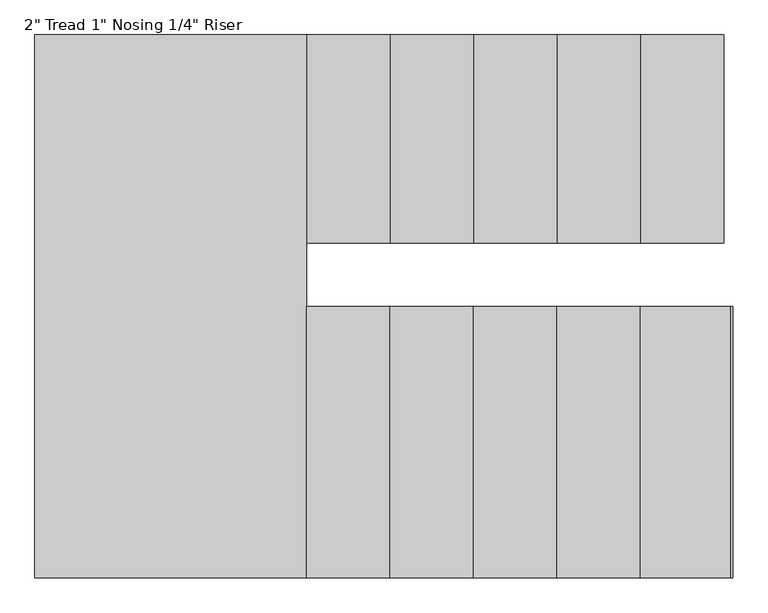
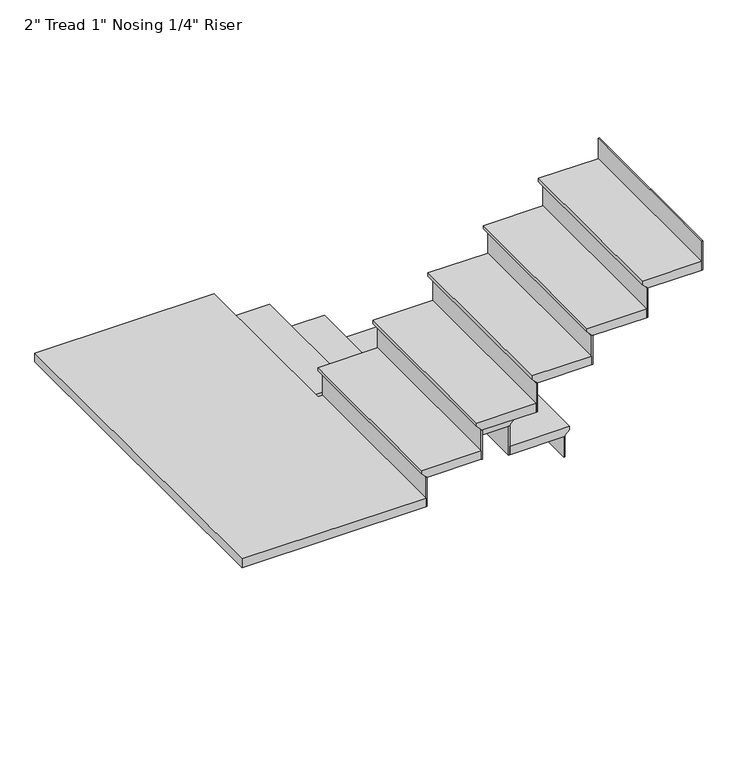
"""IFC4 building model written with IfcOpenShell, lengths in millimetres: stair flight geometry."""

from ifc_helpers import new_model, si_unit, origin, place, context, project, spatial, faceted_brep, source, transform, mapped, element, save


def stair_flight_58fc4bcf(model_context):
    return source(origin(), model_context, "Body", "Brep", [
        faceted_brep([(-3084.0415084, -317.1427733, 6551.0833333), (-3084.0415084, -317.1427733, 6570.1333333), (-3084.0415084, -1076.6758739, 6570.1333333), (-3084.0415084, -1076.6758739, 6551.0833333), (-3109.4415084, -317.1427733, 6525.6833333), (-3109.4415084, -1076.6758739, 6525.6833333), (-3414.2415084, -317.1427733, 6570.1333333), (-3414.2415084, -1076.6758739, 6570.1333333), (-3109.4415084, -1076.6758739, 6519.3333333), (-3414.2415084, -1076.6758739, 6519.3333333), (-3414.2415084, -317.1427733, 6519.3333333), (-3109.4415084, -317.1427733, 6519.3333333)], [[[0, 1, 2, 3]], [[4, 0, 3, 5]], [[2, 1, 6, 7]], [[8, 9, 10, 11]], [[2, 7, 9, 8, 5, 3]], [[8, 11, 4, 5]], [[6, 1, 0, 4, 11, 10]], [[7, 6, 10, 9]]]),
        faceted_brep([(-3109.4415084, -317.1427733, 6519.3333333), (-3109.4415084, -317.1427733, 6400.8), (-3115.7915084, -317.1427733, 6400.8), (-3115.7915084, -317.1427733, 6519.3333333), (-3109.4415084, -1076.6758739, 6519.3333333), (-3115.7915084, -1076.6758739, 6519.3333333), (-3115.7915084, -1076.6758739, 6400.8), (-3109.4415084, -1076.6758739, 6400.8)], [[[0, 1, 2, 3]], [[4, 5, 6, 7]], [[1, 0, 4, 7]], [[2, 1, 7, 6]], [[3, 2, 6, 5]], [[0, 3, 5, 4]]]),
        faceted_brep([(-3414.2415084, -317.1427733, 6688.6666667), (-3414.2415084, -317.1427733, 6519.3333333), (-3420.5915084, -317.1427733, 6519.3333333), (-3420.5915084, -317.1427733, 6688.6666667), (-3414.2415084, -1076.6758739, 6688.6666667), (-3420.5915084, -1076.6758739, 6688.6666667), (-3420.5915084, -1076.6758739, 6519.3333333), (-3414.2415084, -1076.6758739, 6519.3333333)], [[[0, 1, 2, 3]], [[4, 5, 6, 7]], [[1, 0, 4, 7]], [[2, 1, 7, 6]], [[3, 2, 6, 5]], [[0, 3, 5, 4]]]),
        faceted_brep([(-3388.8415084, -1076.6758739, 6739.4666667), (-3388.8415084, -317.1427733, 6739.4666667), (-3719.0415084, -317.1427733, 6739.4666667), (-3719.0415084, -1076.6758739, 6739.4666667), (-3414.2415084, -1076.6758739, 6688.6666667), (-3719.0415084, -1076.6758739, 6688.6666667), (-3719.0415084, -317.1427733, 6688.6666667), (-3414.2415084, -317.1427733, 6688.6666667), (-3414.2415084, -1076.6758739, 6695.0166667), (-3388.8415084, -1076.6758739, 6720.4166667), (-3414.2415084, -317.1427733, 6695.0166667), (-3388.8415084, -317.1427733, 6720.4166667)], [[[0, 1, 2, 3]], [[4, 5, 6, 7]], [[0, 3, 5, 4, 8, 9]], [[4, 7, 10, 8]], [[2, 1, 11, 10, 7, 6]], [[3, 2, 6, 5]], [[11, 1, 0, 9]], [[10, 11, 9, 8]]]),
        faceted_brep([(-3719.0415084, -317.1427733, 6858.0), (-3719.0415084, -317.1427733, 6688.6666667), (-3725.3915084, -317.1427733, 6688.6666667), (-3725.3915084, -317.1427733, 6858.0), (-3719.0415084, -1076.6758739, 6858.0), (-3725.3915084, -1076.6758739, 6858.0), (-3725.3915084, -1076.6758739, 6688.6666667), (-3719.0415084, -1076.6758739, 6688.6666667)], [[[0, 1, 2, 3]], [[4, 5, 6, 7]], [[1, 0, 4, 7]], [[2, 1, 7, 6]], [[3, 2, 6, 5]], [[0, 3, 5, 4]]]),
        faceted_brep([(-3693.6415084, -1076.6758739, 6908.8), (-3693.6415084, -317.1427733, 6908.8), (-4023.8415084, -317.1427733, 6908.8), (-4023.8415084, -1076.6758739, 6908.8), (-3719.0415084, -1076.6758739, 6858.0), (-4023.8415084, -1076.6758739, 6858.0), (-4023.8415084, -317.1427733, 6858.0), (-3719.0415084, -317.1427733, 6858.0), (-3719.0415084, -1076.6758739, 6864.35), (-3693.6415084, -1076.6758739, 6889.75), (-3719.0415084, -317.1427733, 6864.35), (-3693.6415084, -317.1427733, 6889.75)], [[[0, 1, 2, 3]], [[4, 5, 6, 7]], [[0, 3, 5, 4, 8, 9]], [[4, 7, 10, 8]], [[2, 1, 11, 10, 7, 6]], [[3, 2, 6, 5]], [[11, 1, 0, 9]], [[10, 11, 9, 8]]]),
        faceted_brep([(-4023.8415084, -317.1427733, 7027.3333333), (-4023.8415084, -317.1427733, 6858.0), (-4030.1915084, -317.1427733, 6858.0), (-4030.1915084, -317.1427733, 7027.3333333), (-4023.8415084, -1076.6758739, 7027.3333333), (-4030.1915084, -1076.6758739, 7027.3333333), (-4030.1915084, -1076.6758739, 6858.0), (-4023.8415084, -1076.6758739, 6858.0)], [[[0, 1, 2, 3]], [[4, 5, 6, 7]], [[1, 0, 4, 7]], [[2, 1, 7, 6]], [[3, 2, 6, 5]], [[0, 3, 5, 4]]]),
        faceted_brep([(-3998.4415084, -1076.6758739, 7078.1333333), (-3998.4415084, -317.1427733, 7078.1333333), (-4328.6415084, -317.1427733, 7078.1333333), (-4328.6415084, -1076.6758739, 7078.1333333), (-4023.8415084, -1076.6758739, 7027.3333333), (-4328.6415084, -1076.6758739, 7027.3333333), (-4328.6415084, -317.1427733, 7027.3333333), (-4023.8415084, -317.1427733, 7027.3333333), (-4023.8415084, -1076.6758739, 7033.6833333), (-3998.4415084, -1076.6758739, 7059.0833333), (-4023.8415084, -317.1427733, 7033.6833333), (-3998.4415084, -317.1427733, 7059.0833333)], [[[0, 1, 2, 3]], [[4, 5, 6, 7]], [[0, 3, 5, 4, 8, 9]], [[4, 7, 10, 8]], [[2, 1, 11, 10, 7, 6]], [[3, 2, 6, 5]], [[11, 1, 0, 9]], [[10, 11, 9, 8]]]),
        faceted_brep([(-4328.6415084, -317.1427733, 7196.6666667), (-4328.6415084, -317.1427733, 7027.3333333), (-4334.9915084, -317.1427733, 7027.3333333), (-4334.9915084, -317.1427733, 7196.6666667), (-4328.6415084, -1076.6758739, 7196.6666667), (-4334.9915084, -1076.6758739, 7196.6666667), (-4334.9915084, -1076.6758739, 7027.3333333), (-4328.6415084, -1076.6758739, 7027.3333333)], [[[0, 1, 2, 3]], [[4, 5, 6, 7]], [[1, 0, 4, 7]], [[2, 1, 7, 6]], [[3, 2, 6, 5]], [[0, 3, 5, 4]]]),
        faceted_brep([(-4303.2415084, -1076.6758739, 7247.4666667), (-4303.2415084, -317.1427733, 7247.4666667), (-4633.4415084, -317.1427733, 7247.4666667), (-4633.4415084, -1076.6758739, 7247.4666667), (-4328.6415084, -1076.6758739, 7196.6666667), (-4633.4415084, -1076.6758739, 7196.6666667), (-4633.4415084, -317.1427733, 7196.6666667), (-4328.6415084, -317.1427733, 7196.6666667), (-4328.6415084, -1076.6758739, 7203.0166667), (-4303.2415084, -1076.6758739, 7228.4166667), (-4328.6415084, -317.1427733, 7203.0166667), (-4303.2415084, -317.1427733, 7228.4166667)], [[[0, 1, 2, 3]], [[4, 5, 6, 7]], [[0, 3, 5, 4, 8, 9]], [[4, 7, 10, 8]], [[2, 1, 11, 10, 7, 6]], [[3, 2, 6, 5]], [[11, 1, 0, 9]], [[10, 11, 9, 8]]]),
        faceted_brep([(-4633.4415084, -317.1427733, 7366.0), (-4633.4415084, -317.1427733, 7196.6666667), (-4639.7915084, -317.1427733, 7196.6666667), (-4639.7915084, -317.1427733, 7366.0), (-4633.4415084, -1076.6758739, 7366.0), (-4639.7915084, -1076.6758739, 7366.0), (-4639.7915084, -1076.6758739, 7196.6666667), (-4633.4415084, -1076.6758739, 7196.6666667)], [[[0, 1, 2, 3]], [[4, 5, 6, 7]], [[1, 0, 4, 7]], [[2, 1, 7, 6]], [[3, 2, 6, 5]], [[0, 3, 5, 4]]]),
        faceted_brep([(-4582.6415084, -1307.7427733, 7416.8), (-4608.0415084, -1307.7427733, 7416.8), (-4608.0415084, -317.1427733, 7416.8), (-5598.6415084, -317.1427733, 7416.8), (-5598.6415084, -2298.3427733, 7416.8), (-4582.6415084, -2298.3427733, 7416.8), (-4608.0415084, -1307.7427733, 7366.0), (-4582.6415084, -1307.7427733, 7366.0), (-4582.6415084, -2298.3427733, 7366.0), (-5598.6415084, -2298.3427733, 7366.0), (-5598.6415084, -317.1427733, 7366.0), (-4633.4415084, -317.1427733, 7366.0), (-4633.4415084, -1076.6758739, 7366.0), (-4608.0415084, -1076.6758739, 7366.0), (-4608.0415084, -1076.6758739, 7397.75), (-4608.0415084, -317.1427733, 7397.75), (-4633.4415084, -1076.6758739, 7372.35), (-4633.4415084, -317.1427733, 7372.35)], [[[0, 1, 2, 3, 4, 5]], [[6, 7, 8, 9, 10, 11, 12, 13]], [[1, 0, 7, 6]], [[2, 1, 6, 13, 14, 15]], [[13, 12, 16, 14]], [[12, 11, 17, 16]], [[3, 2, 15, 17, 11, 10]], [[4, 3, 10, 9]], [[5, 4, 9, 8]], [[0, 5, 8, 7]], [[17, 15, 14, 16]]]),
        faceted_brep([(-4582.6415084, -2298.3427733, 7535.3333333), (-4582.6415084, -2298.3427733, 7366.0), (-4576.2915084, -2298.3427733, 7366.0), (-4576.2915084, -2298.3427733, 7535.3333333), (-4582.6415084, -1307.7427733, 7535.3333333), (-4576.2915084, -1307.7427733, 7535.3333333), (-4576.2915084, -1307.7427733, 7366.0), (-4582.6415084, -1307.7427733, 7366.0)], [[[0, 1, 2, 3]], [[4, 5, 6, 7]], [[1, 0, 4, 7]], [[2, 1, 7, 6]], [[3, 2, 6, 5]], [[0, 3, 5, 4]]]),
        faceted_brep([(-4608.0415084, -1307.7427733, 7586.1333333), (-4608.0415084, -2298.3427733, 7586.1333333), (-4277.8415084, -2298.3427733, 7586.1333333), (-4277.8415084, -1307.7427733, 7586.1333333), (-4582.6415084, -1307.7427733, 7535.3333333), (-4277.8415084, -1307.7427733, 7535.3333333), (-4277.8415084, -2298.3427733, 7535.3333333), (-4582.6415084, -2298.3427733, 7535.3333333), (-4582.6415084, -1307.7427733, 7541.6833333), (-4608.0415084, -1307.7427733, 7567.0833333), (-4582.6415084, -2298.3427733, 7541.6833333), (-4608.0415084, -2298.3427733, 7567.0833333)], [[[0, 1, 2, 3]], [[4, 5, 6, 7]], [[0, 3, 5, 4, 8, 9]], [[4, 7, 10, 8]], [[2, 1, 11, 10, 7, 6]], [[3, 2, 6, 5]], [[11, 1, 0, 9]], [[10, 11, 9, 8]]]),
        faceted_brep([(-4277.8415084, -2298.3427733, 7704.6666667), (-4277.8415084, -2298.3427733, 7535.3333333), (-4271.4915084, -2298.3427733, 7535.3333333), (-4271.4915084, -2298.3427733, 7704.6666667), (-4277.8415084, -1307.7427733, 7704.6666667), (-4271.4915084, -1307.7427733, 7704.6666667), (-4271.4915084, -1307.7427733, 7535.3333333), (-4277.8415084, -1307.7427733, 7535.3333333)], [[[0, 1, 2, 3]], [[4, 5, 6, 7]], [[1, 0, 4, 7]], [[2, 1, 7, 6]], [[3, 2, 6, 5]], [[0, 3, 5, 4]]]),
        faceted_brep([(-4303.2415084, -1307.7427733, 7755.4666667), (-4303.2415084, -2298.3427733, 7755.4666667), (-3973.0415084, -2298.3427733, 7755.4666667), (-3973.0415084, -1307.7427733, 7755.4666667), (-4277.8415084, -1307.7427733, 7704.6666667), (-3973.0415084, -1307.7427733, 7704.6666667), (-3973.0415084, -2298.3427733, 7704.6666667), (-4277.8415084, -2298.3427733, 7704.6666667), (-4277.8415084, -1307.7427733, 7711.0166667), (-4303.2415084, -1307.7427733, 7736.4166667), (-4277.8415084, -2298.3427733, 7711.0166667), (-4303.2415084, -2298.3427733, 7736.4166667)], [[[0, 1, 2, 3]], [[4, 5, 6, 7]], [[0, 3, 5, 4, 8, 9]], [[4, 7, 10, 8]], [[2, 1, 11, 10, 7, 6]], [[3, 2, 6, 5]], [[11, 1, 0, 9]], [[10, 11, 9, 8]]]),
        faceted_brep([(-3973.0415084, -2298.3427733, 7874.0), (-3973.0415084, -2298.3427733, 7704.6666667), (-3966.6915084, -2298.3427733, 7704.6666667), (-3966.6915084, -2298.3427733, 7874.0), (-3973.0415084, -1307.7427733, 7874.0), (-3966.6915084, -1307.7427733, 7874.0), (-3966.6915084, -1307.7427733, 7704.6666667), (-3973.0415084, -1307.7427733, 7704.6666667)], [[[0, 1, 2, 3]], [[4, 5, 6, 7]], [[1, 0, 4, 7]], [[2, 1, 7, 6]], [[3, 2, 6, 5]], [[0, 3, 5, 4]]]),
        faceted_brep([(-3998.4415084, -1307.7427733, 7924.8), (-3998.4415084, -2298.3427733, 7924.8), (-3668.2415084, -2298.3427733, 7924.8), (-3668.2415084, -1307.7427733, 7924.8), (-3973.0415084, -1307.7427733, 7874.0), (-3668.2415084, -1307.7427733, 7874.0), (-3668.2415084, -2298.3427733, 7874.0), (-3973.0415084, -2298.3427733, 7874.0), (-3973.0415084, -1307.7427733, 7880.35), (-3998.4415084, -1307.7427733, 7905.75), (-3973.0415084, -2298.3427733, 7880.35), (-3998.4415084, -2298.3427733, 7905.75)], [[[0, 1, 2, 3]], [[4, 5, 6, 7]], [[0, 3, 5, 4, 8, 9]], [[4, 7, 10, 8]], [[2, 1, 11, 10, 7, 6]], [[3, 2, 6, 5]], [[11, 1, 0, 9]], [[10, 11, 9, 8]]]),
        faceted_brep([(-3668.2415084, -2298.3427733, 8043.3333333), (-3668.2415084, -2298.3427733, 7874.0), (-3661.8915084, -2298.3427733, 7874.0), (-3661.8915084, -2298.3427733, 8043.3333333), (-3668.2415084, -1307.7427733, 8043.3333333), (-3661.8915084, -1307.7427733, 8043.3333333), (-3661.8915084, -1307.7427733, 7874.0), (-3668.2415084, -1307.7427733, 7874.0)], [[[0, 1, 2, 3]], [[4, 5, 6, 7]], [[1, 0, 4, 7]], [[2, 1, 7, 6]], [[3, 2, 6, 5]], [[0, 3, 5, 4]]]),
        faceted_brep([(-3693.6415084, -1307.7427733, 8094.1333333), (-3693.6415084, -2298.3427733, 8094.1333333), (-3363.4415084, -2298.3427733, 8094.1333333), (-3363.4415084, -1307.7427733, 8094.1333333), (-3668.2415084, -1307.7427733, 8043.3333333), (-3363.4415084, -1307.7427733, 8043.3333333), (-3363.4415084, -2298.3427733, 8043.3333333), (-3668.2415084, -2298.3427733, 8043.3333333), (-3668.2415084, -1307.7427733, 8049.6833333), (-3693.6415084, -1307.7427733, 8075.0833333), (-3668.2415084, -2298.3427733, 8049.6833333), (-3693.6415084, -2298.3427733, 8075.0833333)], [[[0, 1, 2, 3]], [[4, 5, 6, 7]], [[0, 3, 5, 4, 8, 9]], [[4, 7, 10, 8]], [[2, 1, 11, 10, 7, 6]], [[3, 2, 6, 5]], [[11, 1, 0, 9]], [[10, 11, 9, 8]]]),
        faceted_brep([(-3363.4415084, -2298.3427733, 8212.6666667), (-3363.4415084, -2298.3427733, 8043.3333333), (-3357.0915084, -2298.3427733, 8043.3333333), (-3357.0915084, -2298.3427733, 8212.6666667), (-3363.4415084, -1307.7427733, 8212.6666667), (-3357.0915084, -1307.7427733, 8212.6666667), (-3357.0915084, -1307.7427733, 8043.3333333), (-3363.4415084, -1307.7427733, 8043.3333333)], [[[0, 1, 2, 3]], [[4, 5, 6, 7]], [[1, 0, 4, 7]], [[2, 1, 7, 6]], [[3, 2, 6, 5]], [[0, 3, 5, 4]]]),
        faceted_brep([(-3058.6415084, -2298.3427733, 8382.0), (-3058.6415084, -2298.3427733, 8212.6666667), (-3052.2915084, -2298.3427733, 8212.6666667), (-3052.2915084, -2298.3427733, 8382.0), (-3058.6415084, -1307.7427733, 8382.0), (-3052.2915084, -1307.7427733, 8382.0), (-3052.2915084, -1307.7427733, 8212.6666667), (-3058.6415084, -1307.7427733, 8212.6666667)], [[[0, 1, 2, 3]], [[4, 5, 6, 7]], [[1, 0, 4, 7]], [[2, 1, 7, 6]], [[3, 2, 6, 5]], [[0, 3, 5, 4]]]),
        faceted_brep([(-3388.8415084, -1307.7427733, 8263.4666667), (-3388.8415084, -2298.3427733, 8263.4666667), (-3058.6415084, -2298.3427733, 8263.4666667), (-3058.6415084, -1307.7427733, 8263.4666667), (-3363.4415084, -1307.7427733, 8212.6666667), (-3058.6415084, -1307.7427733, 8212.6666667), (-3058.6415084, -2298.3427733, 8212.6666667), (-3363.4415084, -2298.3427733, 8212.6666667), (-3363.4415084, -1307.7427733, 8219.0166667), (-3388.8415084, -1307.7427733, 8244.4166667), (-3363.4415084, -2298.3427733, 8219.0166667), (-3388.8415084, -2298.3427733, 8244.4166667)], [[[0, 1, 2, 3]], [[4, 5, 6, 7]], [[0, 3, 5, 4, 8, 9]], [[4, 7, 10, 8]], [[2, 1, 11, 10, 7, 6]], [[3, 2, 6, 5]], [[11, 1, 0, 9]], [[10, 11, 9, 8]]]),
    ])


if __name__ == "__main__":
    model = new_model("IFC4")
    model_context = context("Model", 3, world=origin())
    ifc_project = project(units=[si_unit("LENGTHUNIT", "METRE", prefix="MILLI")], contexts=[model_context])
    site = spatial("IfcSite", under=ifc_project)
    building = spatial("IfcBuilding", under=site)
    placement = place(None, origin())
    stair_flight_shape = stair_flight_58fc4bcf(model_context)
    element("IfcStairFlight", 1, ObjectType="2\" Tread 1\" Nosing 1/4\" Riser", at=placement, inside=building, context=model_context, shape_type="MappedRepresentation", body=[
        mapped(stair_flight_shape, transform((0.0, 0.0, 0.0), x_axis=(1.0, 0.0, 0.0), y_axis=(0.0, 1.0, 0.0), z_axis=(0.0, 0.0, 1.0))),
    ])
    save(model, "model.ifc")
